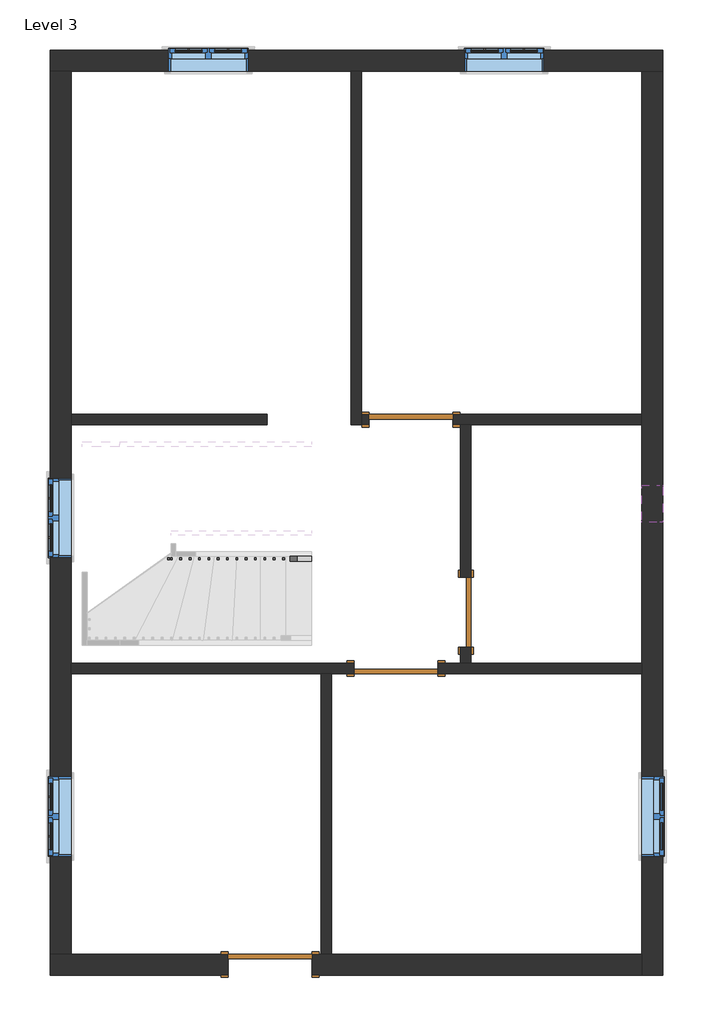
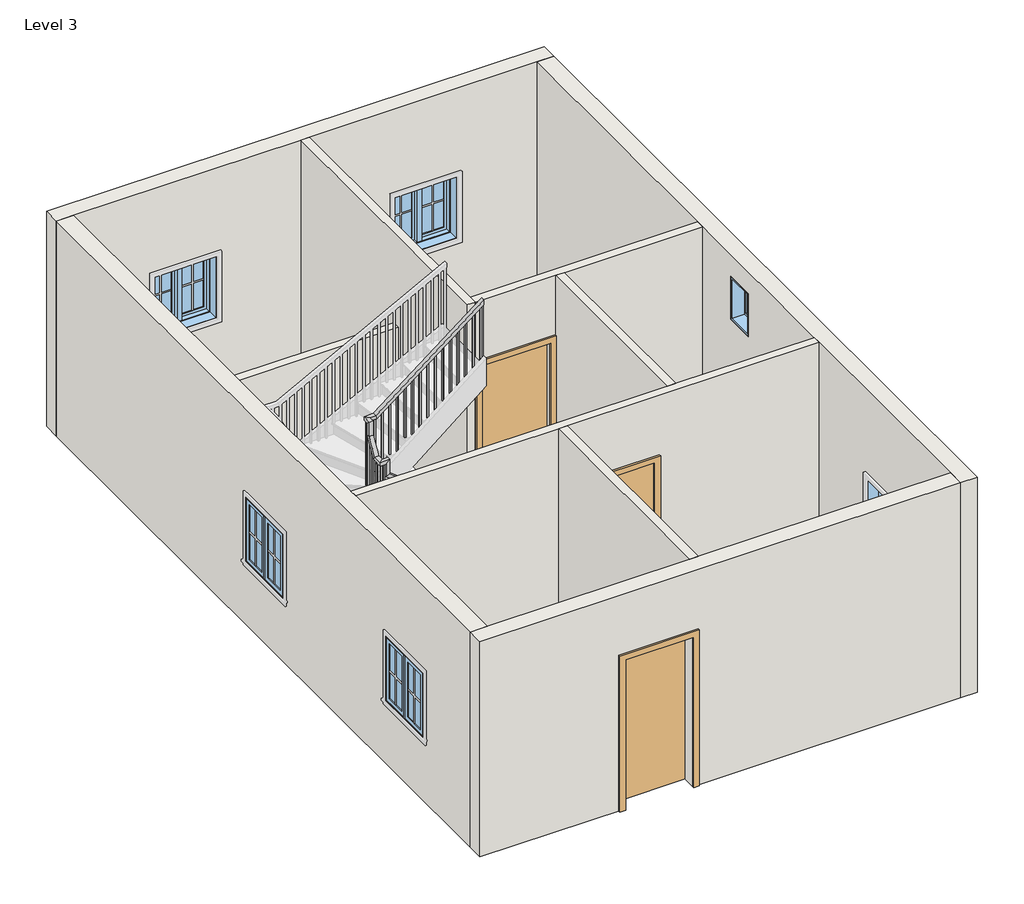
# One storey, part 1 of 2: 10 walls, 6 windows, 4 doors, 1 railing.
"""IFC4 building model written with IfcOpenShell, lengths in millimetres."""

from ifc_helpers import new_model, si_unit, frame, origin, place, context, project, spatial, polyline, outline, extrude, faceted_brep, transform, mapped, element, save
from components import door_d8f5dbb5, door_305aa2a5, door_e5f9f3c4, door_a90ba1ad, window_aa618e30, window_339605e1

model = new_model("IFC4")

# Units and contexts
model_context = context("Model", 3, world=origin())
ifc_project = project(units=[si_unit("LENGTHUNIT", "METRE", prefix="MILLI")], contexts=[model_context])

# Site, building, storey
site = spatial("IfcSite", under=ifc_project)
building = spatial("IfcBuilding", under=site)
storey = spatial("IfcBuildingStorey", under=building, Name="Level 3", Elevation=3200.4)

# Doors
placement = place(None, origin())
door_shape = door_d8f5dbb5(model_context)
element("IfcDoor", 1, ObjectType="Single-Flush : 30\" x 80\"", at=placement, inside=storey, context=model_context, shape_type="MappedRepresentation", body=[
    mapped(door_shape, transform((-82.2715692, -955.3070853, 3200.4), x_axis=(0.0, -1.0, 0.0), y_axis=(1.0, 0.0, 0.0), z_axis=(0.0, 0.0, 1.0))),
])
door_2_shape = door_305aa2a5(model_context)
element("IfcDoor", 2, ObjectType="Single-Flush : 36\" x 84\"", at=placement, inside=storey, context=model_context, shape_type="MappedRepresentation", body=[
    mapped(door_2_shape, transform((-677.5332429, 1140.1929147, 3200.4), x_axis=(-1.0, 0.0, 0.0), y_axis=(0.0, -1.0, 0.0), z_axis=(0.0, 0.0, 1.0))),
])
door_3_shape = door_e5f9f3c4(model_context)
element("IfcDoor", 3, ObjectType="Single-Flush : 36\" x 84\"", at=placement, inside=storey, context=model_context, shape_type="MappedRepresentation", body=[
    mapped(door_3_shape, transform((-842.6332429, -1564.9070853, 3200.4), x_axis=(-1.0, 0.0, 0.0), y_axis=(0.0, -1.0, 0.0), z_axis=(0.0, 0.0, 1.0))),
])
door_4_shape = door_a90ba1ad(model_context)
element("IfcDoor", 4, ObjectType="Single-Flush : 36\" x 84\"", at=placement, inside=storey, context=model_context, shape_type="MappedRepresentation", body=[
    mapped(door_4_shape, transform((-2212.5949167, -4784.3570853, 3200.4), x_axis=(-1.0, 0.0, 0.0), y_axis=(0.0, -1.0, 0.0), z_axis=(0.0, 0.0, 1.0))),
])

# Railing
element("IfcRailing", 5, ObjectType="Handrail - Rectangular", at=placement, inside=storey, context=model_context, shape_type="SolidModel", body=[
    faceted_brep([(-1761.7449167, -396.5070853, 4284.1333333), (-1761.7449167, -396.5070853, 4219.8000346), (-1761.7449167, -345.7070853, 4219.8000346), (-1761.7449167, -345.7070853, 4284.1333333), (-3213.2766085, -396.5070853, 5412.0191036), (-3264.0766085, -396.5070853, 5387.1590024), (-3264.0766085, -345.7070853, 5387.1590024), (-3213.2766085, -345.7070853, 5412.0191036), (-3213.2766085, -396.5070853, 5615.0281882), (-3264.0766085, -396.5070853, 5564.2281882), (-3264.0766085, -345.7070853, 5564.2281882), (-3213.2766085, -345.7070853, 5615.0281882), (-3340.2766085, -396.5070853, 5615.0281882), (-3340.2766085, -396.5070853, 5564.2281882), (-3289.4766085, -345.7070853, 5564.2281882), (-3289.4766085, -345.7070853, 5615.0281882), (-3340.2766085, -269.5070853, 5615.0281882), (-3340.2766085, -240.3857515, 5564.2281882), (-3289.4766085, -240.3857515, 5564.2281882), (-3289.4766085, -269.5070853, 5615.0281882), (-3340.2766085, -142.5070853, 5831.9051451), (-3340.2766085, -91.7070853, 5818.1256424), (-3289.4766085, -91.7070853, 5818.1256424), (-3289.4766085, -142.5070853, 5831.9051451), (-3340.2766085, -142.5070853, 6034.9142297), (-3340.2766085, -91.7070853, 5984.1142297), (-3289.4766085, -91.7070853, 5984.1142297), (-3289.4766085, -142.5070853, 6034.9142297), (-3340.2766085, -15.5070853, 6034.9142297), (-3340.2766085, -15.5070853, 5984.1142297), (-3289.4766085, -66.3070853, 5984.1142297), (-3289.4766085, -66.3070853, 6034.9142297), (-3213.2766085, -15.5070853, 6034.9142297), (-3195.8599406, -15.5070853, 5984.1142297), (-3195.8599406, -66.3070853, 5984.1142297), (-3213.2766085, -66.3070853, 6034.9142297), (-1761.7449167, -15.5070853, 7162.8), (-1761.7449167, -66.3070853, 7162.8), (-1761.7449167, -66.3070853, 7098.4667013), (-1761.7449167, -15.5070853, 7098.4667013)], [[[0, 1, 2, 3]], [[1, 0, 4, 5]], [[2, 1, 5, 6]], [[3, 2, 6, 7]], [[0, 3, 7, 4]], [[5, 4, 8, 9]], [[6, 5, 9, 10]], [[7, 6, 10, 11]], [[4, 7, 11, 8]], [[9, 8, 12, 13]], [[10, 9, 13, 14]], [[11, 10, 14, 15]], [[8, 11, 15, 12]], [[13, 12, 16, 17]], [[14, 13, 17, 18]], [[15, 14, 18, 19]], [[12, 15, 19, 16]], [[17, 16, 20, 21]], [[18, 17, 21, 22]], [[19, 18, 22, 23]], [[16, 19, 23, 20]], [[21, 20, 24, 25]], [[22, 21, 25, 26]], [[23, 22, 26, 27]], [[20, 23, 27, 24]], [[25, 24, 28, 29]], [[26, 25, 29, 30]], [[27, 26, 30, 31]], [[24, 27, 31, 28]], [[29, 28, 32, 33]], [[30, 29, 33, 34]], [[31, 30, 34, 35]], [[28, 31, 35, 32]], [[36, 37, 38, 39]], [[33, 32, 36, 39]], [[34, 33, 39, 38]], [[35, 34, 38, 37]], [[32, 35, 37, 36]]]),
    extrude(outline(polyline([(7083.2316852, -1781.3516085), (7068.4292361, -1800.4016085), (6079.0666667, -1800.4016085), (6079.0666667, -1781.3516085), (7083.2316852, -1781.3516085)])), frame((0.0, -50.4320853, 0.0), z_axis=(0.0, 1.0, 0.0), x_axis=(0.0, 0.0, 1.0)), (0.0, 0.0, 1.0), 19.05),
    extrude(outline(polyline([(7004.2852902, -1882.9516085), (6989.4828411, -1902.0016085), (6079.0666667, -1902.0016085), (6079.0666667, -1882.9516085), (7004.2852902, -1882.9516085)])), frame((0.0, -50.4320853, 0.0), z_axis=(0.0, 1.0, 0.0), x_axis=(0.0, 0.0, 1.0)), (0.0, 0.0, 1.0), 19.05),
    extrude(outline(polyline([(6925.3388952, -1984.5516085), (6910.5364462, -2003.6016085), (6079.0666667, -2003.6016085), (6079.0666667, -1984.5516085), (6925.3388952, -1984.5516085)])), frame((0.0, -50.4320853, 0.0), z_axis=(0.0, 1.0, 0.0), x_axis=(0.0, 0.0, 1.0)), (0.0, 0.0, 1.0), 19.05),
    extrude(outline(polyline([(6846.3925003, -2086.1516085), (6831.5900512, -2105.2016085), (5909.7333333, -2105.2016085), (5909.7333333, -2086.1516085), (6846.3925003, -2086.1516085)])), frame((0.0, -50.4320853, 0.0), z_axis=(0.0, 1.0, 0.0), x_axis=(0.0, 0.0, 1.0)), (0.0, 0.0, 1.0), 19.05),
    extrude(outline(polyline([(6767.4461053, -2187.7516085), (6752.6436562, -2206.8016085), (5909.7333333, -2206.8016085), (5909.7333333, -2187.7516085), (6767.4461053, -2187.7516085)])), frame((0.0, -50.4320853, 0.0), z_axis=(0.0, 1.0, 0.0), x_axis=(0.0, 0.0, 1.0)), (0.0, 0.0, 1.0), 19.05),
    extrude(outline(polyline([(6688.4997103, -2289.3516085), (6673.6972613, -2308.4016085), (5909.7333333, -2308.4016085), (5909.7333333, -2289.3516085), (6688.4997103, -2289.3516085)])), frame((0.0, -50.4320853, 0.0), z_axis=(0.0, 1.0, 0.0), x_axis=(0.0, 0.0, 1.0)), (0.0, 0.0, 1.0), 19.05),
    extrude(outline(polyline([(6609.5533154, -2390.9516085), (6594.7508663, -2410.0016085), (5740.4, -2410.0016085), (5740.4, -2390.9516085), (6609.5533154, -2390.9516085)])), frame((0.0, -50.4320853, 0.0), z_axis=(0.0, 1.0, 0.0), x_axis=(0.0, 0.0, 1.0)), (0.0, 0.0, 1.0), 19.05),
    extrude(outline(polyline([(6530.6069204, -2492.5516085), (6515.8044713, -2511.6016085), (5740.4, -2511.6016085), (5740.4, -2492.5516085), (6530.6069204, -2492.5516085)])), frame((0.0, -50.4320853, 0.0), z_axis=(0.0, 1.0, 0.0), x_axis=(0.0, 0.0, 1.0)), (0.0, 0.0, 1.0), 19.05),
    extrude(outline(polyline([(6451.6605254, -2594.1516085), (6436.8580764, -2613.2016085), (5571.0666667, -2613.2016085), (5571.0666667, -2594.1516085), (6451.6605254, -2594.1516085)])), frame((0.0, -50.4320853, 0.0), z_axis=(0.0, 1.0, 0.0), x_axis=(0.0, 0.0, 1.0)), (0.0, 0.0, 1.0), 19.05),
    extrude(outline(polyline([(6372.7141304, -2695.7516085), (6357.9116814, -2714.8016085), (5571.0666667, -2714.8016085), (5571.0666667, -2695.7516085), (6372.7141304, -2695.7516085)])), frame((0.0, -50.4320853, 0.0), z_axis=(0.0, 1.0, 0.0), x_axis=(0.0, 0.0, 1.0)), (0.0, 0.0, 1.0), 19.05),
    extrude(outline(polyline([(6293.7677355, -2797.3516085), (6278.9652864, -2816.4016085), (5571.0666667, -2816.4016085), (5571.0666667, -2797.3516085), (6293.7677355, -2797.3516085)])), frame((0.0, -50.4320853, 0.0), z_axis=(0.0, 1.0, 0.0), x_axis=(0.0, 0.0, 1.0)), (0.0, 0.0, 1.0), 19.05),
    extrude(outline(polyline([(6214.8213405, -2898.9516085), (6200.0188914, -2918.0016085), (5401.7333333, -2918.0016085), (5401.7333333, -2898.9516085), (6214.8213405, -2898.9516085)])), frame((0.0, -50.4320853, 0.0), z_axis=(0.0, 1.0, 0.0), x_axis=(0.0, 0.0, 1.0)), (0.0, 0.0, 1.0), 19.05),
    extrude(outline(polyline([(6135.8749455, -3000.5516085), (6121.0724965, -3019.6016085), (5401.7333333, -3019.6016085), (5401.7333333, -3000.5516085), (6135.8749455, -3000.5516085)])), frame((0.0, -50.4320853, 0.0), z_axis=(0.0, 1.0, 0.0), x_axis=(0.0, 0.0, 1.0)), (0.0, 0.0, 1.0), 19.05),
    extrude(outline(polyline([(6056.9285506, -3102.1516085), (6042.1261015, -3121.2016085), (5232.4, -3121.2016085), (5232.4, -3102.1516085), (6056.9285506, -3102.1516085)])), frame((0.0, -50.4320853, 0.0), z_axis=(0.0, 1.0, 0.0), x_axis=(0.0, 0.0, 1.0)), (0.0, 0.0, 1.0), 19.05),
    extrude(outline(polyline([(5977.9821556, -3203.7516085), (5963.1797065, -3222.8016085), (5232.4, -3222.8016085), (5232.4, -3203.7516085), (5977.9821556, -3203.7516085)])), frame((0.0, -50.4320853, 0.0), z_axis=(0.0, 1.0, 0.0), x_axis=(0.0, 0.0, 1.0)), (0.0, 0.0, 1.0), 19.05),
    extrude(outline(polyline([(-3305.3516085, -75.8320853), (-3324.4016085, -75.8320853), (-3324.4016085, -56.7820853), (-3305.3516085, -56.7820853), (-3305.3516085, -75.8320853)])), frame((0.0, 0.0, 4893.7333333), z_axis=(0.0, 0.0, 1.0), x_axis=(1.0, 0.0, 0.0)), (0.0, 0.0, 1.0), 1090.3808964),
    extrude(outline(polyline([(-177.4320853, 5671.7336964), (-158.3820853, 5704.26524), (-158.3820853, 4724.4), (-177.4320853, 4724.4), (-177.4320853, 5671.7336964)])), frame((-3324.4016085, 0.0, 0.0), z_axis=(1.0, 0.0, 0.0), x_axis=(0.0, 1.0, 0.0)), (0.0, 0.0, 1.0), 19.05),
    extrude(outline(polyline([(-279.0320853, 5498.2321309), (-259.9820853, 5530.7636744), (-259.9820853, 4555.0666667), (-279.0320853, 4555.0666667), (-279.0320853, 5498.2321309)])), frame((-3324.4016085, 0.0, 0.0), z_axis=(1.0, 0.0, 0.0), x_axis=(0.0, 1.0, 0.0)), (0.0, 0.0, 1.0), 19.05),
    extrude(outline(polyline([(-3276.2199167, -361.5820853), (-3276.2199167, -380.6320853), (-3295.2699167, -380.6320853), (-3295.2699167, -361.5820853), (-3276.2199167, -361.5820853)])), frame((0.0, 0.0, 4385.7333333), z_axis=(0.0, 0.0, 1.0), x_axis=(1.0, 0.0, 0.0)), (0.0, 0.0, 1.0), 1178.4948549),
    extrude(outline(polyline([(5317.6483397, -3174.6199167), (5332.4507888, -3193.6699167), (4216.4, -3193.6699167), (4216.4, -3174.6199167), (5317.6483397, -3174.6199167)])), frame((0.0, -380.6320853, 0.0), z_axis=(0.0, 1.0, 0.0), x_axis=(0.0, 0.0, 1.0)), (0.0, 0.0, 1.0), 19.05),
    extrude(outline(polyline([(5238.7019447, -3073.0199167), (5253.5043938, -3092.0699167), (4216.4, -3092.0699167), (4216.4, -3073.0199167), (5238.7019447, -3073.0199167)])), frame((0.0, -380.6320853, 0.0), z_axis=(0.0, 1.0, 0.0), x_axis=(0.0, 0.0, 1.0)), (0.0, 0.0, 1.0), 19.05),
    extrude(outline(polyline([(5159.7555498, -2971.4199167), (5174.5579988, -2990.4699167), (4047.0666667, -2990.4699167), (4047.0666667, -2971.4199167), (5159.7555498, -2971.4199167)])), frame((0.0, -380.6320853, 0.0), z_axis=(0.0, 1.0, 0.0), x_axis=(0.0, 0.0, 1.0)), (0.0, 0.0, 1.0), 19.05),
    extrude(outline(polyline([(5080.8091548, -2869.8199167), (5095.6116039, -2888.8699167), (4047.0666667, -2888.8699167), (4047.0666667, -2869.8199167), (5080.8091548, -2869.8199167)])), frame((0.0, -380.6320853, 0.0), z_axis=(0.0, 1.0, 0.0), x_axis=(0.0, 0.0, 1.0)), (0.0, 0.0, 1.0), 19.05),
    extrude(outline(polyline([(5001.8627598, -2768.2199167), (5016.6652089, -2787.2699167), (3877.7333333, -2787.2699167), (3877.7333333, -2768.2199167), (5001.8627598, -2768.2199167)])), frame((0.0, -380.6320853, 0.0), z_axis=(0.0, 1.0, 0.0), x_axis=(0.0, 0.0, 1.0)), (0.0, 0.0, 1.0), 19.05),
    extrude(outline(polyline([(4922.9163649, -2666.6199167), (4937.7188139, -2685.6699167), (3877.7333333, -2685.6699167), (3877.7333333, -2666.6199167), (4922.9163649, -2666.6199167)])), frame((0.0, -380.6320853, 0.0), z_axis=(0.0, 1.0, 0.0), x_axis=(0.0, 0.0, 1.0)), (0.0, 0.0, 1.0), 19.05),
    extrude(outline(polyline([(4843.9699699, -2565.0199167), (4858.7724189, -2584.0699167), (3708.4, -2584.0699167), (3708.4, -2565.0199167), (4843.9699699, -2565.0199167)])), frame((0.0, -380.6320853, 0.0), z_axis=(0.0, 1.0, 0.0), x_axis=(0.0, 0.0, 1.0)), (0.0, 0.0, 1.0), 19.05),
    extrude(outline(polyline([(4765.0235749, -2463.4199167), (4779.826024, -2482.4699167), (3708.4, -2482.4699167), (3708.4, -2463.4199167), (4765.0235749, -2463.4199167)])), frame((0.0, -380.6320853, 0.0), z_axis=(0.0, 1.0, 0.0), x_axis=(0.0, 0.0, 1.0)), (0.0, 0.0, 1.0), 19.05),
    extrude(outline(polyline([(4686.0771799, -2361.8199167), (4700.879629, -2380.8699167), (3708.4, -2380.8699167), (3708.4, -2361.8199167), (4686.0771799, -2361.8199167)])), frame((0.0, -380.6320853, 0.0), z_axis=(0.0, 1.0, 0.0), x_axis=(0.0, 0.0, 1.0)), (0.0, 0.0, 1.0), 19.05),
    extrude(outline(polyline([(4607.130785, -2260.2199167), (4621.933234, -2279.2699167), (3539.0666667, -2279.2699167), (3539.0666667, -2260.2199167), (4607.130785, -2260.2199167)])), frame((0.0, -380.6320853, 0.0), z_axis=(0.0, 1.0, 0.0), x_axis=(0.0, 0.0, 1.0)), (0.0, 0.0, 1.0), 19.05),
    extrude(outline(polyline([(4528.18439, -2158.6199167), (4542.9868391, -2177.6699167), (3539.0666667, -2177.6699167), (3539.0666667, -2158.6199167), (4528.18439, -2158.6199167)])), frame((0.0, -380.6320853, 0.0), z_axis=(0.0, 1.0, 0.0), x_axis=(0.0, 0.0, 1.0)), (0.0, 0.0, 1.0), 19.05),
    extrude(outline(polyline([(4449.237995, -2057.0199167), (4464.0404441, -2076.0699167), (3539.0666667, -2076.0699167), (3539.0666667, -2057.0199167), (4449.237995, -2057.0199167)])), frame((0.0, -380.6320853, 0.0), z_axis=(0.0, 1.0, 0.0), x_axis=(0.0, 0.0, 1.0)), (0.0, 0.0, 1.0), 19.05),
    extrude(outline(polyline([(4370.2916001, -1955.4199167), (4385.0940491, -1974.4699167), (3369.7333333, -1974.4699167), (3369.7333333, -1955.4199167), (4370.2916001, -1955.4199167)])), frame((0.0, -380.6320853, 0.0), z_axis=(0.0, 1.0, 0.0), x_axis=(0.0, 0.0, 1.0)), (0.0, 0.0, 1.0), 19.05),
    extrude(outline(polyline([(4291.3452051, -1853.8199167), (4306.1476541, -1872.8699167), (3369.7333333, -1872.8699167), (3369.7333333, -1853.8199167), (4291.3452051, -1853.8199167)])), frame((0.0, -380.6320853, 0.0), z_axis=(0.0, 1.0, 0.0), x_axis=(0.0, 0.0, 1.0)), (0.0, 0.0, 1.0), 19.05),
    extrude(outline(polyline([(-3305.3516085, -50.4320853), (-3324.4016085, -50.4320853), (-3324.4016085, -31.3820853), (-3305.3516085, -31.3820853), (-3305.3516085, -50.4320853)])), frame((0.0, 0.0, 5063.0666667), z_axis=(0.0, 0.0, 1.0), x_axis=(1.0, 0.0, 0.0)), (0.0, 0.0, 1.0), 921.0475631),
    extrude(outline(polyline([(-3305.3516085, -361.5820853), (-3305.3516085, -380.6320853), (-3324.4016085, -380.6320853), (-3324.4016085, -361.5820853), (-3305.3516085, -361.5820853)])), frame((0.0, 0.0, 4385.7333333), z_axis=(0.0, 0.0, 1.0), x_axis=(1.0, 0.0, 0.0)), (0.0, 0.0, 1.0), 1178.4948549),
    extrude(outline(polyline([(7098.4667013, -1761.7449167), (7083.6642523, -1780.7949167), (6079.0666667, -1780.7949167), (6079.0666667, -1761.7449167), (7098.4667013, -1761.7449167)])), frame((0.0, -50.4320853, 0.0), z_axis=(0.0, 1.0, 0.0), x_axis=(0.0, 0.0, 1.0)), (0.0, 0.0, 1.0), 19.05),
    extrude(outline(polyline([(4219.8000346, -1761.7449167), (4234.6024837, -1780.7949167), (3369.7333333, -1780.7949167), (3369.7333333, -1761.7449167), (4219.8000346, -1761.7449167)])), frame((0.0, -380.6320853, 0.0), z_axis=(0.0, 1.0, 0.0), x_axis=(0.0, 0.0, 1.0)), (0.0, 0.0, 1.0), 19.05),
])

# Walls
element("IfcWall", 6, ObjectType="WALL4.5\"", at=placement, inside=storey, context=model_context, shape_type="Brep", body=[
    faceted_brep([(-1329.9449167, 4931.1429147, 3200.4), (-1329.9449167, 1083.0429147, 3200.4), (-1329.9449167, 1083.0429147, 6248.4), (-1329.9449167, 4931.1429147, 6248.4), (-1215.6449167, 4931.1429147, 3200.4), (-1215.6449167, 4931.1429147, 6248.4), (-1215.6449167, 1197.3429147, 6248.4), (-1215.6449167, 1083.0429147, 6248.4), (-1215.6449167, 1083.0429147, 3200.4), (-1215.6449167, 1197.3429147, 3200.4)], [[[0, 1, 2, 3]], [[4, 5, 6, 7, 8, 9]], [[1, 0, 4, 9, 8]], [[0, 3, 5, 4]], [[2, 1, 8, 7]], [[3, 2, 7, 6, 5]]]),
])
element("IfcWall", 7, ObjectType="WALL4.5\"", at=placement, inside=storey, context=model_context, shape_type="Brep", body=[
    faceted_brep([(-1215.6449167, 1083.0429147, 3200.4), (-1134.7332429, 1083.0429147, 3200.4), (-1134.7332429, 1083.0429147, 5334.0), (-220.3332429, 1083.0429147, 5334.0), (-220.3332429, 1083.0429147, 3200.4), (-139.4215692, 1083.0429147, 3200.4), (-25.1215692, 1083.0429147, 3200.4), (1832.3550833, 1083.0429147, 3200.4), (1832.3550833, 1083.0429147, 6248.4), (-25.1215692, 1083.0429147, 6248.4), (-139.4215692, 1083.0429147, 6248.4), (-1215.6449167, 1083.0429147, 6248.4), (-1134.7332429, 1197.3429147, 5334.0), (-1134.7332429, 1197.3429147, 3200.4), (-1215.6449167, 1197.3429147, 3200.4), (-1215.6449167, 1197.3429147, 6248.4), (1832.3550833, 1197.3429147, 6248.4), (1832.3550833, 1197.3429147, 3200.4), (-220.3332429, 1197.3429147, 3200.4), (-220.3332429, 1197.3429147, 5334.0)], [[[0, 1, 2, 3, 4, 5, 6, 7, 8, 9, 10, 11]], [[12, 13, 14, 15, 16, 17, 18, 19]], [[18, 17, 7, 6, 5, 4]], [[14, 13, 1, 0]], [[0, 11, 15, 14]], [[8, 7, 17, 16]], [[2, 1, 13, 12]], [[3, 2, 12, 19]], [[4, 3, 19, 18]], [[11, 10, 9, 8, 16, 15]]]),
])
element("IfcWall", 8, ObjectType="WALL4.5\"", at=placement, inside=storey, context=model_context, shape_type="SweptSolid", body=[
    extrude(outline(polyline([(-2244.3449167, 1083.0429147), (-4377.9449167, 1083.0429147), (-4377.9449167, 1197.3429147), (-2244.3449167, 1197.3429147), (-2244.3449167, 1083.0429147)])), frame((0.0, 0.0, 3200.4), z_axis=(0.0, 0.0, 1.0), x_axis=(1.0, 0.0, 0.0)), (0.0, 0.0, 1.0), 3048.0),
])
element("IfcWall", 9, ObjectType="WALL4.5\"", at=placement, inside=storey, context=model_context, shape_type="SweptSolid", body=[
    extrude(outline(polyline([(-1336.3070853, 5232.4), (-1336.3070853, 3200.4), (-1507.7570853, 3200.4), (-1507.7570853, 6248.4), (1083.0429147, 6248.4), (1083.0429147, 3200.4), (-574.3070853, 3200.4), (-574.3070853, 5232.4), (-1336.3070853, 5232.4)])), frame((-139.4215692, 0.0, 0.0), z_axis=(1.0, 0.0, 0.0), x_axis=(0.0, 1.0, 0.0)), (0.0, 0.0, 1.0), 114.3),
])
element("IfcWall", 10, ObjectType="WALL4.5\"", at=placement, inside=storey, context=model_context, shape_type="Brep", body=[
    faceted_brep([(-4377.9449167, -1622.0570853, 3200.4), (-1660.1449167, -1622.0570853, 3200.4), (-1545.8449167, -1622.0570853, 3200.4), (-1299.8332429, -1622.0570853, 3200.4), (-1299.8332429, -1622.0570853, 5334.0), (-385.4332429, -1622.0570853, 5334.0), (-385.4332429, -1622.0570853, 3200.4), (1832.3550833, -1622.0570853, 3200.4), (1832.3550833, -1622.0570853, 6248.4), (-1545.8449167, -1622.0570853, 6248.4), (-1660.1449167, -1622.0570853, 6248.4), (-4377.9449167, -1622.0570853, 6248.4), (-1299.8332429, -1507.7570853, 5334.0), (-1299.8332429, -1507.7570853, 3200.4), (-4377.9449167, -1507.7570853, 3200.4), (-4377.9449167, -1507.7570853, 6248.4), (-139.4215692, -1507.7570853, 6248.4), (-25.1215692, -1507.7570853, 6248.4), (1832.3550833, -1507.7570853, 6248.4), (1832.3550833, -1507.7570853, 3200.4), (-25.1215692, -1507.7570853, 3200.4), (-139.4215692, -1507.7570853, 3200.4), (-385.4332429, -1507.7570853, 3200.4), (-385.4332429, -1507.7570853, 5334.0)], [[[0, 1, 2, 3, 4, 5, 6, 7, 8, 9, 10, 11]], [[12, 13, 14, 15, 16, 17, 18, 19, 20, 21, 22, 23]], [[14, 13, 3, 2, 1, 0]], [[22, 21, 20, 19, 7, 6]], [[8, 7, 19, 18]], [[0, 11, 15, 14]], [[4, 3, 13, 12]], [[5, 4, 12, 23]], [[6, 5, 23, 22]], [[11, 10, 9, 8, 18, 17, 16, 15]]]),
])
element("IfcWall", 11, ObjectType="WALL4.5\"", at=placement, inside=storey, context=model_context, shape_type="SweptSolid", body=[
    extrude(outline(polyline([(-1660.1449167, -4670.0570853), (-1660.1449167, -1622.0570853), (-1545.8449167, -1622.0570853), (-1545.8449167, -4670.0570853), (-1660.1449167, -4670.0570853)])), frame((0.0, 0.0, 3200.4), z_axis=(0.0, 0.0, 1.0), x_axis=(1.0, 0.0, 0.0)), (0.0, 0.0, 1.0), 3048.0),
])
element("IfcWall", 12, ObjectType="WALL9\"", at=placement, inside=storey, context=model_context, shape_type="Brep", body=[
    faceted_brep([(-4606.5449167, 4931.1429147, 3200.4), (-4377.9449167, 4931.1429147, 3200.4), (-1329.9449167, 4931.1429147, 3200.4), (-1215.6449167, 4931.1429147, 3200.4), (1832.3550833, 4931.1429147, 3200.4), (2060.9550833, 4931.1429147, 3200.4), (2060.9550833, 4931.1429147, 6248.4), (1832.3550833, 4931.1429147, 6248.4), (-1215.6449167, 4931.1429147, 6248.4), (-1329.9449167, 4931.1429147, 6248.4), (-4377.9449167, 4931.1429147, 6248.4), (-4606.5449167, 4931.1429147, 6248.4), (-2450.7199167, 4931.1429147, 5029.2), (-2450.7199167, 4931.1429147, 4114.8), (-3314.3199167, 4931.1429147, 4114.8), (-3314.3199167, 4931.1429147, 5029.2), (768.7300833, 4931.1429147, 5029.2), (768.7300833, 4931.1429147, 4114.8), (-94.8699167, 4931.1429147, 4114.8), (-94.8699167, 4931.1429147, 5029.2), (-4606.5449167, 5159.7429147, 3200.4), (-4606.5449167, 5159.7429147, 6248.4), (2060.9550833, 5159.7429147, 6248.4), (2060.9550833, 5159.7429147, 3200.4), (-2450.7199167, 5159.7429147, 5029.2), (-3314.3199167, 5159.7429147, 5029.2), (-3314.3199167, 5159.7429147, 4114.8), (-2450.7199167, 5159.7429147, 4114.8), (768.7300833, 5159.7429147, 5029.2), (-94.8699167, 5159.7429147, 5029.2), (-94.8699167, 5159.7429147, 4114.8), (768.7300833, 5159.7429147, 4114.8)], [[[0, 1, 2, 3, 4, 5, 6, 7, 8, 9, 10, 11], [12, 13, 14, 15], [16, 17, 18, 19]], [[20, 21, 22, 23], [24, 25, 26, 27], [28, 29, 30, 31]], [[5, 4, 3, 2, 1, 0, 20, 23]], [[6, 5, 23, 22]], [[0, 11, 21, 20]], [[13, 12, 24, 27]], [[14, 13, 27, 26]], [[15, 14, 26, 25]], [[12, 15, 25, 24]], [[17, 16, 28, 31]], [[18, 17, 31, 30]], [[19, 18, 30, 29]], [[16, 19, 29, 28]], [[11, 10, 9, 8, 7, 6, 22, 21]]]),
])
element("IfcWall", 13, ObjectType="WALL9\"", at=placement, inside=storey, context=model_context, shape_type="Brep", body=[
    faceted_brep([(1832.3550833, 4931.1429147, 3200.4), (1832.3550833, 1197.3429147, 3200.4), (1832.3550833, 1083.0429147, 3200.4), (1832.3550833, -1507.7570853, 3200.4), (1832.3550833, -1622.0570853, 3200.4), (1832.3550833, -4670.0570853, 3200.4), (1832.3550833, -4898.6570853, 3200.4), (1832.3550833, -4898.6570853, 6248.4), (1832.3550833, -4670.0570853, 6248.4), (1832.3550833, -1622.0570853, 6248.4), (1832.3550833, -1507.7570853, 6248.4), (1832.3550833, 1083.0429147, 6248.4), (1832.3550833, 1197.3429147, 6248.4), (1832.3550833, 4931.1429147, 6248.4), (1832.3550833, 22.5929147, 5943.6), (1832.3550833, 22.5929147, 5334.0), (1832.3550833, 428.9929147, 5334.0), (1832.3550833, 428.9929147, 5943.6), (1832.3550833, -3606.4320853, 5029.2), (1832.3550833, -3606.4320853, 4114.8), (1832.3550833, -2742.8320853, 4114.8), (1832.3550833, -2742.8320853, 5029.2), (2060.9550833, 4931.1429147, 3200.4), (2060.9550833, 4931.1429147, 6248.4), (2060.9550833, -4898.6570853, 6248.4), (2060.9550833, -4898.6570853, 3200.4), (2060.9550833, 22.5929147, 5943.6), (2060.9550833, 428.9929147, 5943.6), (2060.9550833, 428.9929147, 5334.0), (2060.9550833, 22.5929147, 5334.0), (2060.9550833, -3606.4320853, 5029.2), (2060.9550833, -2742.8320853, 5029.2), (2060.9550833, -2742.8320853, 4114.8), (2060.9550833, -3606.4320853, 4114.8)], [[[0, 1, 2, 3, 4, 5, 6, 7, 8, 9, 10, 11, 12, 13], [14, 15, 16, 17], [18, 19, 20, 21]], [[22, 23, 24, 25], [26, 27, 28, 29], [30, 31, 32, 33]], [[6, 5, 4, 3, 2, 1, 0, 22, 25]], [[0, 13, 23, 22]], [[7, 6, 25, 24]], [[15, 14, 26, 29]], [[16, 15, 29, 28]], [[17, 16, 28, 27]], [[14, 17, 27, 26]], [[19, 18, 30, 33]], [[20, 19, 33, 32]], [[21, 20, 32, 31]], [[18, 21, 31, 30]], [[13, 12, 11, 10, 9, 8, 7, 24, 23]]]),
])
element("IfcWall", 14, ObjectType="WALL9\"", at=placement, inside=storey, context=model_context, shape_type="Brep", body=[
    faceted_brep([(-2669.7949167, -4670.0570853, 5334.0), (-2669.7949167, -4670.0570853, 3200.4), (-4377.9449167, -4670.0570853, 3200.4), (-4606.5449167, -4670.0570853, 3200.4), (-4606.5449167, -4670.0570853, 6248.4), (-4377.9449167, -4670.0570853, 6248.4), (-1660.1449167, -4670.0570853, 6248.4), (-1545.8449167, -4670.0570853, 6248.4), (1832.3550833, -4670.0570853, 6248.4), (1832.3550833, -4670.0570853, 3200.4), (-1545.8449167, -4670.0570853, 3200.4), (-1660.1449167, -4670.0570853, 3200.4), (-1755.3949167, -4670.0570853, 3200.4), (-1755.3949167, -4670.0570853, 5334.0), (-4606.5449167, -4898.6570853, 3200.4), (-2669.7949167, -4898.6570853, 3200.4), (-2669.7949167, -4898.6570853, 5334.0), (-1755.3949167, -4898.6570853, 5334.0), (-1755.3949167, -4898.6570853, 3200.4), (1832.3550833, -4898.6570853, 3200.4), (1832.3550833, -4898.6570853, 6248.4), (-4606.5449167, -4898.6570853, 6248.4)], [[[0, 1, 2, 3, 4, 5, 6, 7, 8, 9, 10, 11, 12, 13]], [[14, 15, 16, 17, 18, 19, 20, 21]], [[3, 2, 1, 15, 14]], [[12, 11, 10, 9, 19, 18]], [[9, 8, 20, 19]], [[4, 3, 14, 21]], [[16, 15, 1, 0]], [[17, 16, 0, 13]], [[18, 17, 13, 12]], [[8, 7, 6, 5, 4, 21, 20]]]),
])
element("IfcWall", 15, ObjectType="WALL9\"", at=placement, inside=storey, context=model_context, shape_type="Brep", body=[
    faceted_brep([(-4377.9449167, -4670.0570853, 3200.4), (-4377.9449167, -1622.0570853, 3200.4), (-4377.9449167, -1507.7570853, 3200.4), (-4377.9449167, 1083.0429147, 3200.4), (-4377.9449167, 1197.3429147, 3200.4), (-4377.9449167, 4931.1429147, 3200.4), (-4377.9449167, 4931.1429147, 6248.4), (-4377.9449167, 1197.3429147, 6248.4), (-4377.9449167, 1083.0429147, 6248.4), (-4377.9449167, -1507.7570853, 6248.4), (-4377.9449167, -1622.0570853, 6248.4), (-4377.9449167, -4670.0570853, 6248.4), (-4377.9449167, -2742.8320853, 5029.2), (-4377.9449167, -2742.8320853, 4114.8), (-4377.9449167, -3606.4320853, 4114.8), (-4377.9449167, -3606.4320853, 5029.2), (-4377.9449167, 505.1929147, 5029.2), (-4377.9449167, 505.1929147, 4114.8), (-4377.9449167, -358.4070853, 4114.8), (-4377.9449167, -358.4070853, 5029.2), (-4606.5449167, -4670.0570853, 3200.4), (-4606.5449167, -4670.0570853, 6248.4), (-4606.5449167, 4931.1429147, 6248.4), (-4606.5449167, 4931.1429147, 3200.4), (-4606.5449167, -2742.8320853, 5029.2), (-4606.5449167, -3606.4320853, 5029.2), (-4606.5449167, -3606.4320853, 4114.8), (-4606.5449167, -2742.8320853, 4114.8), (-4606.5449167, 505.1929147, 5029.2), (-4606.5449167, -358.4070853, 5029.2), (-4606.5449167, -358.4070853, 4114.8), (-4606.5449167, 505.1929147, 4114.8)], [[[0, 1, 2, 3, 4, 5, 6, 7, 8, 9, 10, 11], [12, 13, 14, 15], [16, 17, 18, 19]], [[20, 21, 22, 23], [24, 25, 26, 27], [28, 29, 30, 31]], [[5, 4, 3, 2, 1, 0, 20, 23]], [[0, 11, 21, 20]], [[6, 5, 23, 22]], [[13, 12, 24, 27]], [[14, 13, 27, 26]], [[15, 14, 26, 25]], [[12, 15, 25, 24]], [[17, 16, 28, 31]], [[18, 17, 31, 30]], [[19, 18, 30, 29]], [[16, 19, 29, 28]], [[11, 10, 9, 8, 7, 6, 22, 21]]]),
])

# Windows
window_shape = window_aa618e30(model_context)
element("IfcWindow", 16, ObjectType="Fixed : 16\" x 24\"", at=placement, inside=storey, context=model_context, shape_type="MappedRepresentation", body=[
    mapped(window_shape, transform((1946.6550833, 187.6929147, 4419.6), x_axis=(0.0, -1.0, 0.0), y_axis=(1.0, 0.0, 0.0), z_axis=(0.0, 0.0, 1.0))),
])
window_2_shape = window_339605e1(model_context)
element("IfcWindow", 17, ObjectType="Window-Casement-Double : 34\" x 36\"", at=placement, inside=storey, context=model_context, shape_type="MappedRepresentation", body=[
    mapped(window_2_shape, transform((-2882.5199167, 5045.4429147, 3200.4), x_axis=(1.0, 0.0, 0.0), y_axis=(0.0, 1.0, 0.0), z_axis=(0.0, 0.0, 1.0))),
])
element("IfcWindow", 18, ObjectType="Window-Casement-Double : 34\" x 36\"", at=placement, inside=storey, context=model_context, shape_type="MappedRepresentation", body=[
    mapped(window_2_shape, transform((336.9300833, 5045.4429147, 3200.4), x_axis=(1.0, 0.0, 0.0), y_axis=(0.0, 1.0, 0.0), z_axis=(0.0, 0.0, 1.0))),
])
element("IfcWindow", 19, ObjectType="Window-Casement-Double : 34\" x 36\"", at=placement, inside=storey, context=model_context, shape_type="MappedRepresentation", body=[
    mapped(window_2_shape, transform((-4492.2449167, -3174.6320853, 3200.4), x_axis=(0.0, 1.0, 0.0), y_axis=(-1.0, 0.0, 0.0), z_axis=(0.0, 0.0, 1.0))),
])
element("IfcWindow", 20, ObjectType="Window-Casement-Double : 34\" x 36\"", at=placement, inside=storey, context=model_context, shape_type="MappedRepresentation", body=[
    mapped(window_2_shape, transform((1946.6550833, -3174.6320853, 3200.4), x_axis=(0.0, -1.0, 0.0), y_axis=(1.0, 0.0, 0.0), z_axis=(0.0, 0.0, 1.0))),
])
element("IfcWindow", 21, ObjectType="Window-Casement-Double : 34\" x 36\"", at=placement, inside=storey, context=model_context, shape_type="MappedRepresentation", body=[
    mapped(window_2_shape, transform((-4492.2449167, 73.3929147, 3200.4), x_axis=(0.0, 1.0, 0.0), y_axis=(-1.0, 0.0, 0.0), z_axis=(0.0, 0.0, 1.0))),
])

save(model, "model.ifc")

# Revit data of these elements
# Type "Single-Flush : 30\" x 80\""
#   Type Mark = "5"
#   Construction Type Id = "MDOOR"
#   Assembly Code = "C1020"
#   Analytic Construction = "Metal"
#   Thickness = 0' - 2"
#   Heat Transfer Coefficient (U) = 0.651978 BTU/(h·ft²·°F)
#   Height = 6' - 8"
#   Trim Projection Ext = 0' - 1"
#   Trim Projection Int = 0' - 1"
#   Trim Width = 0' - 3"
#   Width = 2' - 6"
#   Define Thermal Properties by = 1
#   Define Thermal Properties by = 1
#   Door Material = Door - Panel
#   Frame Material = Door - Frame
#   Visual Light Transmittance = 0
#   Solar Heat Gain Coefficient = 0
#   Function = (empty or 0)
#   Wall Closure = (empty or 0)
# Type "Single-Flush : 36\" x 84\""
#   Type Mark = "1"
#   Construction Type Id = "MDOOR"
#   Assembly Code = "C1020"
#   Analytic Construction = "Metal"
#   Thickness = 0' - 2"
#   Heat Transfer Coefficient (U) = 0.651978 BTU/(h·ft²·°F)
#   Height = 7' - 0"
#   Trim Projection Ext = 0' - 1"
#   Trim Projection Int = 0' - 1"
#   Trim Width = 0' - 3"
#   Width = 3' - 0"
#   Define Thermal Properties by = 1
#   Define Thermal Properties by = 1
#   Door Material = Door - Panel
#   Frame Material = Door - Frame
#   Visual Light Transmittance = 0
#   Solar Heat Gain Coefficient = 0
#   Function = (empty or 0)
#   Wall Closure = (empty or 0)
# Type "Handrail - Rectangular"
#   Assembly Code = "C2010400"
#   built-in parameter 1008612 = 0.0416667 (stored number, unit not read)
#   built-in parameter 1008611 = 0.0416667 (stored number, unit not read)
#   built-in parameter 1008609 = 0.333333 (stored number, unit not read)
#   built-in parameter 1008604 = 0.166667 (stored number, unit not read)
#   built-in parameter 1008603 = 0.166667 (stored number, unit not read)
#   Railing Height = 3' - 0"
#   built-in parameter 1008630 = 2
#   built-in parameter 1008610 = 2
#   built-in parameter 1008618 = Baluster - Square : 3/4"
# Type "WALL4.5\""
#   Assembly Code = "B2010"
#   Layers, outside or top first: 0' - 4 1/2" no material (function 1)
# Type "WALL9\""
#   Assembly Code = "B2010"
#   Layers, outside or top first: 0' - 9" no material (function 1)
# Type "Fixed : 16\" x 24\""
#   Type Mark = "4"
#   Construction Type Id = "GSP4R"
#   Assembly Code = "B2020100"
#   Analytic Construction = "1/8 in Pilkington single glazing"
#   Visual Light Transmittance = 0.9
#   Solar Heat Gain Coefficient = 0.78
#   Heat Transfer Coefficient (U) = 0.6496 BTU/(h·ft²·°F)
#   Height = 2' - 0"
#   Default Sill Height = 3' - 0"
#   Width = 1' - 4"
#   Window Inset = 0' - 0 3/4"
#   Define Thermal Properties by = 1
#   Define Thermal Properties by = 1
#   Glass Pane Material = Glass
#   Sash Material = Sash
#   Wall Closure = (empty or 0)
# Type "Window-Casement-Double : 34\" x 36\""
#   Type Mark = "14"
#   Fire Rating = "0.5h"
#   Assembly Code = "B2020100"
#   Analytic Construction = "Double glazing - domestic"
#   Frame Extension [instance default] = 0' - 0 1/4"
#   Window Inset [instance default] = 0' - 0"
#   Wall Thickness [instance default] = 0' - 6"
#   Interior Wall Closure [instance default] = 0' - 2 1/4"
#   Half Width = 1' - 5"
#   Visual Light Transmittance = 0.81
#   Thermal Resistance (R) = 1.8146 (h·ft²·°F)/BTU
#   Solar Heat Gain Coefficient = 0.76
#   Rough Width = 2' - 10 1/2"
#   Rough Height = 3' - 0 1/2"
#   Height = 3' - 0"
#   Heat Transfer Coefficient (U) = 0.5511 BTU/(h·ft²·°F)
#   Exterior Wall Closure [instance default] = 0' - 1 1/4"
#   Extension Jamb [instance default] = 0' - 2 1/4"
#   Default Sill Height = 3' - 0"
#   Width = 2' - 10"
#   Define Thermal Properties by = 0
#   Muntin Visibility = yes
#   Interior Trim Visibility [instance default] = yes
#   Exterior Trim Visibility [instance default] = yes
#   Extension Jamb Visibility [instance default] = yes
#   Interior Trim Material = Wood - Stained
#   Muntin Pattern = Muntin Pattern_2x2 : Muntin Pattern_2x2
#   Interior Trim = Trim-Window-Interior-Flat : Picture Frame
#   Interior Frame Material = Wood - Stained
#   Glass Panel Material = Glass
#   Exterior Trim Material = Clad - White
#   Exterior Trim = Trim-Window-Exterior-Flat : with Sill
#   Exterior Frame Material = Clad - White
#   Wall Closure = (empty or 0)
# Element 1 (IfcDoor, "Single-Flush : 30\" x 80\"")
#   Phase Created = New Construction
#   Materials on its faces: "Door - Frame", "Door - Panel"
# Elements 2, 3, 4 (IfcDoor, "Single-Flush : 36\" x 84\"")
#   Phase Created = New Construction
#   Materials on its faces: "Door - Frame", "Door - Panel"
# Element 5 (IfcRailing, "Handrail - Rectangular")
#   Phase Created = New Construction
# Elements 6, 7, 8, 9, 10, 11 (IfcWall, "WALL4.5\"")
#   Top Offset = 0' - 0"
#   Base Offset = 0' - 0"
#   Unconnected Height = 10' - 0"
#   wall height = 10' - 0"
#   Phase Created = New Construction
#   Base Constraint = Level 3
#   Materials on its faces: "Default Wall"
# Elements 12, 13, 14, 15 (IfcWall, "WALL9\"")
#   Top Offset = 0' - 0"
#   Base Offset = 0' - 0"
#   Unconnected Height = 10' - 0"
#   wall height = 10' - 0"
#   Phase Created = New Construction
#   Base Constraint = Level 3
#   Materials on its faces: "Default Wall", "Brick, Soldier Course"
# Element 16 (IfcWindow, "Fixed : 16\" x 24\"")
#   Mark = "7"
#   Phase Created = New Construction
#   Materials on its faces: "Sash", "Glass"
# Element 17 (IfcWindow, "Window-Casement-Double : 34\" x 36\"")
#   Mark = "8"
#   Window Inset = 0' - 0"
#   Interior Wall Closure = 0' - 2 1/4"
#   Frame Extension = 0' - 0 1/4"
#   Exterior Wall Closure = 0' - 1 1/4"
#   Interior Trim Visibility = yes
#   Exterior Trim Visibility = yes
#   Phase Created = New Construction
#   Materials on its faces: "Wood - Stained", "Glass", "Clad - White"
# Element 18 (IfcWindow, "Window-Casement-Double : 34\" x 36\"")
#   Mark = "9"
#   Window Inset = 0' - 0"
#   Interior Wall Closure = 0' - 2 1/4"
#   Frame Extension = 0' - 0 1/4"
#   Exterior Wall Closure = 0' - 1 1/4"
#   Interior Trim Visibility = yes
#   Exterior Trim Visibility = yes
#   Phase Created = New Construction
#   Materials on its faces: "Wood - Stained", "Glass", "Clad - White"
# Element 19 (IfcWindow, "Window-Casement-Double : 34\" x 36\"")
#   Mark = "10"
#   Window Inset = 0' - 0"
#   Interior Wall Closure = 0' - 2 1/4"
#   Frame Extension = 0' - 0 1/4"
#   Exterior Wall Closure = 0' - 1 1/4"
#   Interior Trim Visibility = yes
#   Exterior Trim Visibility = yes
#   Phase Created = New Construction
#   Materials on its faces: "Wood - Stained", "Glass", "Clad - White"
# Element 20 (IfcWindow, "Window-Casement-Double : 34\" x 36\"")
#   Mark = "11"
#   Window Inset = 0' - 0"
#   Interior Wall Closure = 0' - 2 1/4"
#   Frame Extension = 0' - 0 1/4"
#   Exterior Wall Closure = 0' - 1 1/4"
#   Interior Trim Visibility = yes
#   Exterior Trim Visibility = yes
#   Phase Created = New Construction
#   Materials on its faces: "Wood - Stained", "Glass", "Clad - White"
# Element 21 (IfcWindow, "Window-Casement-Double : 34\" x 36\"")
#   Mark = "12"
#   Window Inset = 0' - 0"
#   Interior Wall Closure = 0' - 2 1/4"
#   Frame Extension = 0' - 0 1/4"
#   Exterior Wall Closure = 0' - 1 1/4"
#   Interior Trim Visibility = yes
#   Exterior Trim Visibility = yes
#   Phase Created = New Construction
#   Materials on its faces: "Wood - Stained", "Glass", "Clad - White"
# Materials
#   "Door - Panel": class "Wood", colour RGB 210 159 95, transparency 0, Cost = 0
#   "Door - Frame": colour RGB 118 70 51, transparency 0, Cost = 0
#   "Glass": class "Glass", colour RGB 0 128 192, transparency 0.75, Description = "Soda Lime Glass", Cost = 0
#   "Sash": class "Wood", colour RGB 224 178 126, transparency 0, Cost = 0
#   "Wood - Stained": class "Wood", colour RGB 224 178 126, transparency 0, Cost = 0
#   "Clad - White": class "Wood", colour RGB 242 242 238, transparency 0, Cost = 0
#   "Default Wall": colour RGB 128 128 128, transparency 0, Cost = 0
#   "Brick, Soldier Course": class "Masonry", colour RGB 170 98 104, transparency 0, Description = "Common brick soldier coursed", Cost = 0
